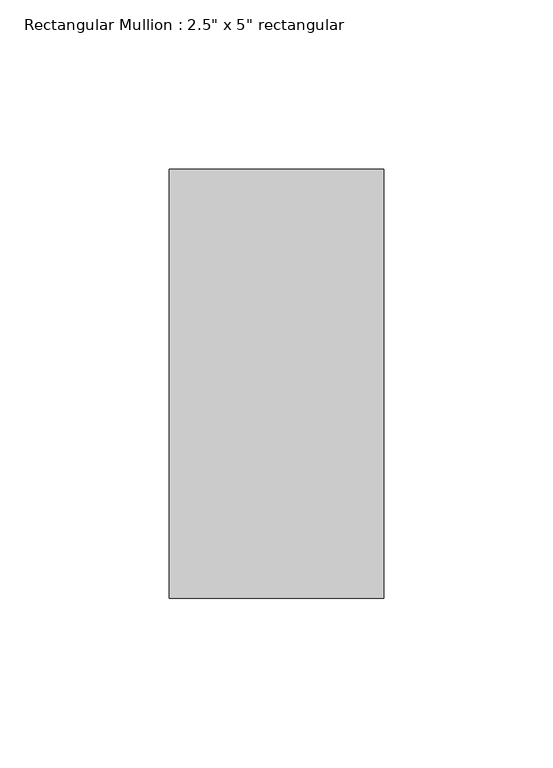
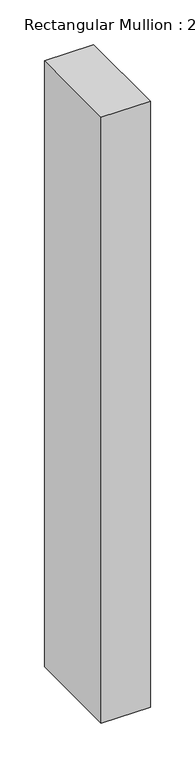
"""IFC4 building model written with IfcOpenShell, lengths in millimetres: member geometry."""

from ifc_helpers import new_model, si_unit, frame, origin, place, context, project, spatial, polyline, outline, extrude, source, transform, mapped, element, save


def member_4df5bd8f(model_context):
    return source(origin(), model_context, "Body", "SweptSolid", [
        extrude(outline(polyline([(0.0, 63.5), (0.0, -63.5), (-63.5, -63.5), (-63.5, 63.5), (0.0, 63.5)])), frame((0.0, 0.0, -827.3309713), z_axis=(0.0, 0.0, 1.0), x_axis=(1.0, 0.0, 0.0)), (0.0, 0.0, 1.0), 827.3309713),
    ])


if __name__ == "__main__":
    model = new_model("IFC4")
    model_context = context("Model", 3, world=origin())
    ifc_project = project(units=[si_unit("LENGTHUNIT", "METRE", prefix="MILLI")], contexts=[model_context])
    site = spatial("IfcSite", under=ifc_project)
    building = spatial("IfcBuilding", under=site)
    placement = place(None, origin())
    member_shape = member_4df5bd8f(model_context)
    element("IfcMember", 1, ObjectType="Rectangular Mullion : 2.5\" x 5\" rectangular", at=placement, inside=building, context=model_context, shape_type="MappedRepresentation", body=[
        mapped(member_shape, transform((0.0, 0.0, 0.0), x_axis=(1.0, 0.0, 0.0), y_axis=(0.0, 1.0, 0.0), z_axis=(0.0, 0.0, 1.0))),
    ])
    save(model, "model.ifc")

# Revit data of these elements
# Type "Rectangular Mullion : 2.5\" x 5\" rectangular"
#   built-in parameter 1007304 = 0.416667 (stored number, unit not read)
#   built-in parameter 1007301 = 0.104167 (stored number, unit not read)
#   built-in parameter 1007300 = 0.104167 (stored number, unit not read)
# Element 1 (IfcMember, "Rectangular Mullion : 2.5\" x 5\" rectangular")
#   Materials on its faces: "Aluminum"
# Materials
#   "Aluminum": class "Metal", colour RGB 247 247 247, transparency 0, Description = "Aluminum 6061", Cost = 0
